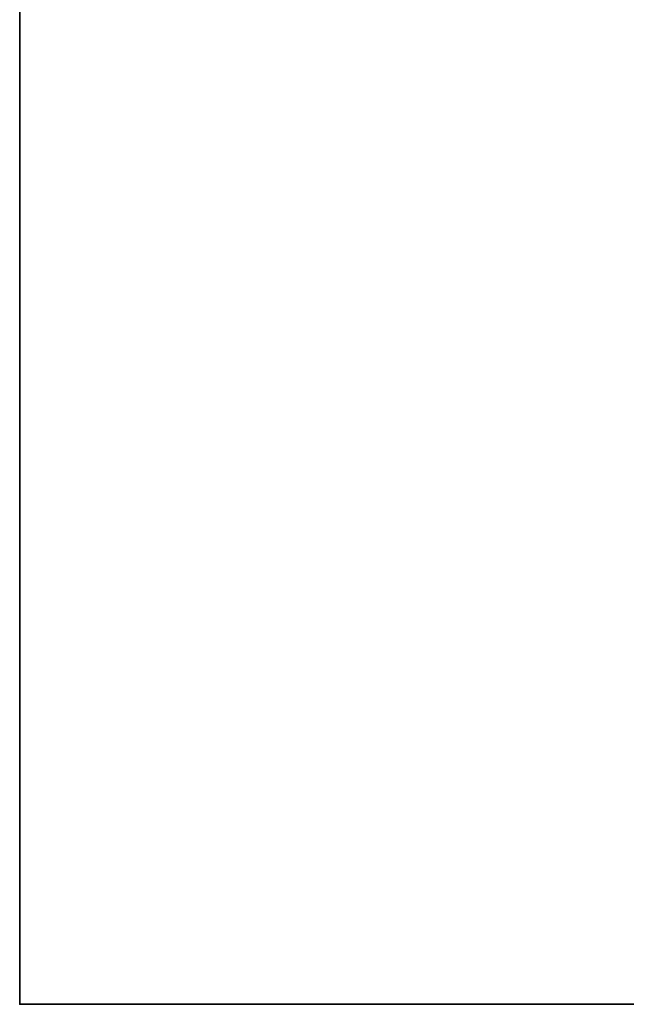
# Model space of a CAD drawing. Units: inches. Extents: x -31485 to -28799, y 18003 to 19130.
# Tile 1 of 15: x -31485 to -31242, y 18003 to 18398. Entities that reach past the tile are written whole.
import ezdxf

# ---------------------------------------------------------------- set-up
doc = ezdxf.new("R2010")
doc.units = ezdxf.units.IN
doc.layers.add('A-ANNO-TTLB', color=7, linetype='Continuous', lineweight=35)

msp = doc.modelspace()

# ---------------------------------------------------------------- linework, layer by layer
at = {"layer": 'A-ANNO-TTLB'}
msp.add_lwpolyline([(-31485.09529421644, 19129.94040955191), (-28798.6381181599, 19129.94040955191), (-28798.6381181599, 18002.86338091846), (-31485.09529421644, 18002.86338091846)], close=True, dxfattribs=at)

doc.saveas('drawing.dxf')
